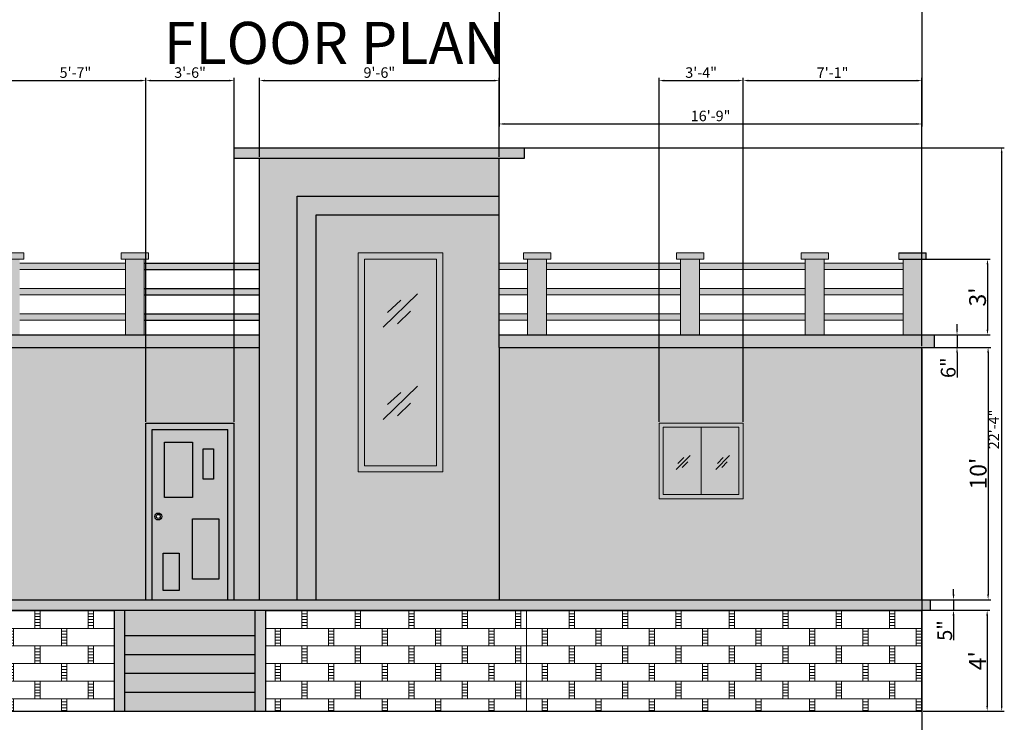
# Model space of a CAD drawing. Units: inches. Extents: x 1662 to 23131, y 1265 to 19127.
# Tile 23 of 26: x 22111 to 22579, y 18027 to 18361. Entities that reach past the tile are written whole.
import ezdxf

# ---------------------------------------------------------------- set-up
doc = ezdxf.new("R2010")
doc.units = ezdxf.units.IN
for name, color, linetype, lineweight in [('A-ANNO-DIMS', 4, 'Continuous', 18), ('A-ANNO-TITL', 7, 'Continuous', 35), ('A-ELEV', 7, 'Continuous', 25), ('A-ELEV-GLAZ', 4, 'Continuous', 18), ('A-ELEV-PATT', 8, 'Continuous', 13), ('A-ELEV-RAIL', 7, 'Continuous', 18), ('A-ELEV-SURF-PATT', 252, 'Continuous', 13)]:
    doc.layers.add(name, color=color, linetype=linetype, lineweight=lineweight)
doc.styles.get("Standard").update_dxf_attribs({"font": 'arial.ttf'})
doc.dimstyles.new('ISO-25', dxfattribs={"dimtxt": 5, "dimasz": 2.5, "dimexe": 1.25, "dimexo": 0.625, "dimtad": 1, "dimlunit": 3, "dimtxsty": 'Standard', "dimcen": 2.5, "dimadec": 0, "dimazin": 0, "dimtfac": 1, "dimtmove": 0, "dimatfit": 3, "dimfxl": 1, "dimarcsym": 0})

# ---------------------------------------------------------------- blocks, each defined once
blk = doc.blocks.new('*D137')
at = {"layer": 'A-ANNO-DIMS', "color": 0, "lineweight": -2, "transparency": 16777216}
for p, q in [((22540.77, 18080.22), (22572.4, 18080.22)), ((22571.15, 18077.72), (22571.15, 18034.72)), ((22540.77, 18032.22), (22572.4, 18032.22))]:
    blk.add_line(p, q, dxfattribs=at)
at = {"layer": 'A-ANNO-DIMS', "color": 0, "transparency": 16777216}
for points in [[(22570.74, 18077.72), (22571.57, 18077.72), (22571.15, 18080.22)], [(22570.74, 18034.72), (22571.57, 18034.72), (22571.15, 18032.22)]]:
    blk.add_solid(points, dxfattribs=at)
at = {"layer": 'Defpoints', "color": 0, "transparency": 16777216}
for p in [(22540.15, 18080.22), (22540.15, 18032.22), (22571.15, 18032.22)]:
    blk.add_point(p, dxfattribs=at)
at = {"layer": 'A-ANNO-DIMS', "color": 0, "transparency": 16777216, "insert": (22566.53, 18056.22), "char_height": 5, "attachment_point": 5, "rotation": 90}
blk.add_mtext("{\\H1.6x;4'}", dxfattribs=at)
blk = doc.blocks.new('*D138')
at = {"layer": 'A-ANNO-DIMS', "color": 0, "lineweight": -2, "transparency": 16777216}
for p, q in [((22555.15, 18087.72), (22555.15, 18090.22)), ((22544.77, 18085.22), (22556.4, 18085.22)), ((22555.15, 18085.22), (22555.15, 18080.22)), ((22544.77, 18080.22), (22556.4, 18080.22)), ((22555.15, 18077.72), (22555.15, 18065.93))]:
    blk.add_line(p, q, dxfattribs=at)
at = {"layer": 'A-ANNO-DIMS', "color": 0, "transparency": 16777216}
for points in [[(22554.73, 18087.72), (22555.57, 18087.72), (22555.15, 18085.22)], [(22554.73, 18077.72), (22555.57, 18077.72), (22555.15, 18080.22)]]:
    blk.add_solid(points, dxfattribs=at)
at = {"layer": 'Defpoints', "color": 0, "transparency": 16777216}
for p in [(22544.15, 18085.22), (22544.15, 18080.22), (22555.15, 18080.22)]:
    blk.add_point(p, dxfattribs=at)
at = {"layer": 'A-ANNO-DIMS', "color": 0, "transparency": 16777216, "insert": (22550.97, 18070.57), "char_height": 5, "attachment_point": 5, "rotation": 90}
blk.add_mtext('{\\H1.4x;5"}', dxfattribs=at)
blk = doc.blocks.new('*D139')
at = {"layer": 'A-ANNO-DIMS', "color": 0, "lineweight": -2, "transparency": 16777216}
for p, q in [((22540.77, 18205.22), (22572.85, 18205.22)), ((22571.6, 18202.72), (22571.6, 18087.72)), ((22540.77, 18085.22), (22572.85, 18085.22))]:
    blk.add_line(p, q, dxfattribs=at)
at = {"layer": 'A-ANNO-DIMS', "color": 0, "transparency": 16777216}
for points in [[(22571.18, 18202.72), (22572.02, 18202.72), (22571.6, 18205.22)], [(22571.18, 18087.72), (22572.02, 18087.72), (22571.6, 18085.22)]]:
    blk.add_solid(points, dxfattribs=at)
at = {"layer": 'Defpoints', "color": 0, "transparency": 16777216}
for p in [(22540.15, 18205.22), (22540.15, 18085.22), (22571.6, 18085.22)]:
    blk.add_point(p, dxfattribs=at)
at = {"layer": 'A-ANNO-DIMS', "color": 0, "transparency": 16777216, "insert": (22566.89, 18145.22), "char_height": 5, "attachment_point": 5, "rotation": 90}
blk.add_mtext("{\\H1.6x;10'}", dxfattribs=at)
blk = doc.blocks.new('*D140')
at = {"layer": 'A-ANNO-DIMS', "color": 0, "lineweight": -2, "transparency": 16777216}
for p, q in [((22556.81, 18213.72), (22556.81, 18216.22)), ((22546.77, 18211.22), (22558.06, 18211.22)), ((22556.81, 18211.22), (22556.81, 18205.22)), ((22546.77, 18205.22), (22558.06, 18205.22)), ((22556.81, 18202.72), (22556.81, 18190.89))]:
    blk.add_line(p, q, dxfattribs=at)
at = {"layer": 'A-ANNO-DIMS', "color": 0, "transparency": 16777216}
for points in [[(22556.4, 18213.72), (22557.23, 18213.72), (22556.81, 18211.22)], [(22556.4, 18202.72), (22557.23, 18202.72), (22556.81, 18205.22)]]:
    blk.add_solid(points, dxfattribs=at)
at = {"layer": 'Defpoints', "color": 0, "transparency": 16777216}
for p in [(22546.15, 18211.22), (22546.15, 18205.22), (22556.81, 18205.22)]:
    blk.add_point(p, dxfattribs=at)
at = {"layer": 'A-ANNO-DIMS', "color": 0, "transparency": 16777216, "insert": (22552.61, 18195.56), "char_height": 5, "attachment_point": 5, "rotation": 90}
blk.add_mtext('{\\H1.4x;6"}', dxfattribs=at)
blk = doc.blocks.new('*D141')
at = {"layer": 'A-ANNO-DIMS', "color": 0, "lineweight": -2, "transparency": 16777216}
for p, q in [((22540.77, 18247.22), (22572.55, 18247.22)), ((22571.3, 18244.72), (22571.3, 18213.72)), ((22540.77, 18211.22), (22572.55, 18211.22))]:
    blk.add_line(p, q, dxfattribs=at)
at = {"layer": 'A-ANNO-DIMS', "color": 0, "transparency": 16777216}
for points in [[(22570.88, 18244.72), (22571.71, 18244.72), (22571.3, 18247.22)], [(22570.88, 18213.72), (22571.71, 18213.72), (22571.3, 18211.22)]]:
    blk.add_solid(points, dxfattribs=at)
at = {"layer": 'Defpoints', "color": 0, "transparency": 16777216}
for p in [(22540.15, 18247.22), (22540.15, 18211.22), (22571.3, 18211.22)]:
    blk.add_point(p, dxfattribs=at)
at = {"layer": 'A-ANNO-DIMS', "color": 0, "transparency": 16777216, "insert": (22566.58, 18229.22), "char_height": 5, "attachment_point": 5, "rotation": 90}
blk.add_mtext("{\\H1.6x;3'}", dxfattribs=at)
blk = doc.blocks.new('GLAZ-REFLECTION')
for p, q in [((0, 0), (6.63, 6.69)), ((0.83, 2.91), (3.6, 5.77)), ((2.93, 0.98), (5.5, 3.58))]:
    blk.add_line(p, q)
blk = doc.blocks.new('*D255')
at = {"layer": 'A-ANNO-DIMS', "color": 0, "lineweight": -2, "transparency": 16777216}
for p, q in [((22339.15, 18570.08), (22339.15, 18310.24)), ((22540.15, 18570.08), (22540.15, 18310.24)), ((22341.65, 18311.49), (22537.65, 18311.49))]:
    blk.add_line(p, q, dxfattribs=at)
at = {"layer": 'A-ANNO-DIMS', "color": 0, "transparency": 16777216}
for points in [[(22341.65, 18311.91), (22341.65, 18311.08), (22339.15, 18311.49)], [(22537.65, 18311.91), (22537.65, 18311.08), (22540.15, 18311.49)]]:
    blk.add_solid(points, dxfattribs=at)
at = {"layer": 'Defpoints', "color": 0, "transparency": 16777216}
for p in [(22339.15, 18570.71), (22540.15, 18570.71), (22540.15, 18311.49)]:
    blk.add_point(p, dxfattribs=at)
at = {"layer": 'A-ANNO-DIMS', "color": 0, "transparency": 16777216, "insert": (22439.65, 18314.67), "char_height": 5, "attachment_point": 5}
blk.add_mtext('16\'-9"', dxfattribs=at)
blk = doc.blocks.new('*D257')
at = {"layer": 'A-ANNO-DIMS', "color": 0, "lineweight": -2, "transparency": 16777216}
for p, q in [((21988.15, 18204.6), (21988.15, 17831.29)), ((22540.15, 18204.6), (22540.15, 17831.29)), ((21990.65, 17832.54), (22537.65, 17832.54))]:
    blk.add_line(p, q, dxfattribs=at)
at = {"layer": 'A-ANNO-DIMS', "color": 0, "transparency": 16777216}
for points in [[(21990.65, 17832.96), (21990.65, 17832.12), (21988.15, 17832.54)], [(22537.65, 17832.96), (22537.65, 17832.12), (22540.15, 17832.54)]]:
    blk.add_solid(points, dxfattribs=at)
at = {"layer": 'Defpoints', "color": 0, "transparency": 16777216}
for p in [(21988.15, 18205.22), (22540.15, 18205.22), (22540.15, 17832.54)]:
    blk.add_point(p, dxfattribs=at)
at = {"layer": 'A-ANNO-DIMS', "color": 0, "transparency": 16777216, "insert": (22264.15, 17835.72), "char_height": 5, "attachment_point": 5}
blk.add_mtext('46\'-0"', dxfattribs=at)
blk = doc.blocks.new('*D258')
at = {"layer": 'A-ANNO-DIMS', "color": 0, "lineweight": -2, "transparency": 16777216}
for p, q in [((22213.77, 18300.22), (22579.3, 18300.22)), ((22578.05, 18034.72), (22578.05, 18297.72)), ((22540.77, 18032.22), (22579.3, 18032.22))]:
    blk.add_line(p, q, dxfattribs=at)
at = {"layer": 'A-ANNO-DIMS', "color": 0, "transparency": 16777216}
for points in [[(22577.63, 18297.72), (22578.47, 18297.72), (22578.05, 18300.22)], [(22577.63, 18034.72), (22578.47, 18034.72), (22578.05, 18032.22)]]:
    blk.add_solid(points, dxfattribs=at)
at = {"layer": 'Defpoints', "color": 0, "transparency": 16777216}
for p in [(22213.15, 18300.22), (22578.05, 18300.22), (22540.15, 18032.22)]:
    blk.add_point(p, dxfattribs=at)
at = {"layer": 'A-ANNO-DIMS', "color": 0, "transparency": 16777216, "insert": (22574.91, 18166.22), "char_height": 5, "attachment_point": 5, "rotation": 90}
blk.add_mtext('22\'-4"', dxfattribs=at)
blk = doc.blocks.new('*D261')
at = {"layer": 'A-ANNO-DIMS', "color": 0, "lineweight": -2, "transparency": 16777216}
for p, q in [((22104.15, 18169.85), (22104.15, 18333.37)), ((22171.15, 18169.85), (22171.15, 18333.37)), ((22106.65, 18332.12), (22168.65, 18332.12))]:
    blk.add_line(p, q, dxfattribs=at)
at = {"layer": 'A-ANNO-DIMS', "color": 0, "transparency": 16777216}
for points in [[(22106.65, 18332.54), (22106.65, 18331.71), (22104.15, 18332.12)], [(22168.65, 18332.54), (22168.65, 18331.71), (22171.15, 18332.12)]]:
    blk.add_solid(points, dxfattribs=at)
at = {"layer": 'Defpoints', "color": 0, "transparency": 16777216}
for p in [(22171.15, 18332.12), (22104.15, 18169.22), (22171.15, 18169.22)]:
    blk.add_point(p, dxfattribs=at)
at = {"layer": 'A-ANNO-DIMS', "color": 0, "transparency": 16777216, "insert": (22137.65, 18335.29), "char_height": 5, "attachment_point": 5}
blk.add_mtext('5\'-7"', dxfattribs=at)
blk = doc.blocks.new('*D262')
at = {"layer": 'A-ANNO-DIMS', "color": 0, "lineweight": -2, "transparency": 16777216}
for p, q in [((22171.15, 18169.85), (22171.15, 18333.37)), ((22213.15, 18169.85), (22213.15, 18333.37)), ((22173.65, 18332.12), (22210.65, 18332.12))]:
    blk.add_line(p, q, dxfattribs=at)
at = {"layer": 'A-ANNO-DIMS', "color": 0, "transparency": 16777216}
for points in [[(22173.65, 18332.54), (22173.65, 18331.71), (22171.15, 18332.12)], [(22210.65, 18332.54), (22210.65, 18331.71), (22213.15, 18332.12)]]:
    blk.add_solid(points, dxfattribs=at)
at = {"layer": 'Defpoints', "color": 0, "transparency": 16777216}
for p in [(22213.15, 18332.12), (22171.15, 18169.22), (22213.15, 18169.22)]:
    blk.add_point(p, dxfattribs=at)
at = {"layer": 'A-ANNO-DIMS', "color": 0, "transparency": 16777216, "insert": (22192.15, 18335.3), "char_height": 5, "attachment_point": 5}
blk.add_mtext('3\'-6"', dxfattribs=at)
blk = doc.blocks.new('*D263')
at = {"layer": 'A-ANNO-DIMS', "color": 0, "lineweight": -2, "transparency": 16777216}
for p, q in [((22225.15, 18295.85), (22225.15, 18333.37)), ((22339.15, 18295.85), (22339.15, 18333.37)), ((22227.65, 18332.12), (22336.65, 18332.12))]:
    blk.add_line(p, q, dxfattribs=at)
at = {"layer": 'A-ANNO-DIMS', "color": 0, "transparency": 16777216}
for points in [[(22227.65, 18332.54), (22227.65, 18331.71), (22225.15, 18332.12)], [(22336.65, 18332.54), (22336.65, 18331.71), (22339.15, 18332.12)]]:
    blk.add_solid(points, dxfattribs=at)
at = {"layer": 'Defpoints', "color": 0, "transparency": 16777216}
for p in [(22339.15, 18332.12), (22225.15, 18295.22), (22339.15, 18295.22)]:
    blk.add_point(p, dxfattribs=at)
at = {"layer": 'A-ANNO-DIMS', "color": 0, "transparency": 16777216, "insert": (22282.15, 18335.3), "char_height": 5, "attachment_point": 5}
blk.add_mtext('9\'-6"', dxfattribs=at)
blk = doc.blocks.new('*D264')
at = {"layer": 'A-ANNO-DIMS', "color": 0, "lineweight": -2, "transparency": 16777216}
for p, q in [((22415.15, 18169.85), (22415.15, 18333.37)), ((22455.15, 18169.85), (22455.15, 18333.37)), ((22417.65, 18332.12), (22452.65, 18332.12))]:
    blk.add_line(p, q, dxfattribs=at)
at = {"layer": 'A-ANNO-DIMS', "color": 0, "transparency": 16777216}
for points in [[(22417.65, 18332.54), (22417.65, 18331.71), (22415.15, 18332.12)], [(22452.65, 18332.54), (22452.65, 18331.71), (22455.15, 18332.12)]]:
    blk.add_solid(points, dxfattribs=at)
at = {"layer": 'Defpoints', "color": 0, "transparency": 16777216}
for p in [(22455.15, 18332.12), (22415.15, 18169.22), (22455.15, 18169.22)]:
    blk.add_point(p, dxfattribs=at)
at = {"layer": 'A-ANNO-DIMS', "color": 0, "transparency": 16777216, "insert": (22435.15, 18335.3), "char_height": 5, "attachment_point": 5}
blk.add_mtext('3\'-4"', dxfattribs=at)
blk = doc.blocks.new('*D265')
at = {"layer": 'A-ANNO-DIMS', "color": 0, "lineweight": -2, "transparency": 16777216}
for p, q in [((22455.15, 18169.85), (22455.15, 18333.37)), ((22540.15, 18205.85), (22540.15, 18333.37)), ((22457.65, 18332.12), (22537.65, 18332.12))]:
    blk.add_line(p, q, dxfattribs=at)
at = {"layer": 'A-ANNO-DIMS', "color": 0, "transparency": 16777216}
for points in [[(22457.65, 18332.54), (22457.65, 18331.71), (22455.15, 18332.12)], [(22537.65, 18332.54), (22537.65, 18331.71), (22540.15, 18332.12)]]:
    blk.add_solid(points, dxfattribs=at)
at = {"layer": 'Defpoints', "color": 0, "transparency": 16777216}
for p in [(22540.15, 18332.12), (22540.15, 18205.22), (22455.15, 18169.22)]:
    blk.add_point(p, dxfattribs=at)
at = {"layer": 'A-ANNO-DIMS', "color": 0, "transparency": 16777216, "insert": (22497.65, 18335.26), "char_height": 5, "attachment_point": 5}
blk.add_mtext('7\'-1"', dxfattribs=at)

msp = doc.modelspace()

# ---------------------------------------------------------------- hatches: boundary and pattern name
at = {"layer": 'A-ELEV-PATT'}
h = msp.add_hatch(dxfattribs=at)
h.set_pattern_fill('BRSTONE', color=256)
h.paths.add_polyline_path([(22156.149, 18080.223), (22079.649, 18080.223), (22079.649, 18032.223), (22156.149, 18032.223)])
h.paths.add_polyline_path([(22079.649, 18080.223), (22048.849, 18080.223), (22049.648, 18077.151), (22046.197, 18075.676), (22049.648, 18074.202), (22051.373, 18060.93), (22047.922, 18055.032), (22052.523, 18054.294), (22053.673, 18052.082), (22050.798, 18046.921), (22055.399, 18043.972), (22050.798, 18039.548), (22053.673, 18039.548), (22058.118, 18032.223), (22079.649, 18032.223)])
h.paths.add_polyline_path([(21997.887, 18071.252), (22000.763, 18076.413), (22004.213, 18077.151), (22004.746, 18080.223), (21988.149, 18080.223), (21988.149, 18042.556), (21991.561, 18047.659), (21992.711, 18055.032), (21990.986, 18056.506), (21994.436, 18064.617), (21998.462, 18065.354)])
h = msp.add_hatch(dxfattribs=at)
h.set_pattern_fill('AR-BRSTD', color=256)
h.paths.add_polyline_path([(22339.149, 18080.223), (22228.149, 18080.223), (22228.149, 18032.223), (22339.149, 18032.223)])
h.paths.add_polyline_path([(22540.149, 18080.223), (22339.149, 18080.223), (22339.149, 18032.223), (22540.149, 18032.223)])
h = msp.add_hatch(dxfattribs=at)
h.set_pattern_fill('AR-BRSTD', color=256)
h.paths.add_polyline_path([(22540.149, 18080.223), (22228.149, 18080.223), (22228.149, 18032.223), (22540.149, 18032.223)])
h = msp.add_hatch(dxfattribs=at)
h.set_pattern_fill('BRSTONE', color=256)
h.paths.add_polyline_path([(22540.149, 18080.223), (22228.149, 18080.223), (22228.149, 18032.223), (22540.149, 18032.223)])
at = {"layer": 'A-ELEV-SURF-PATT'}
h = msp.add_hatch(color=256, dxfattribs=at)
h.dxf.hatch_style = 1
h.paths.add_polyline_path([(22225.149, 18211.223), (21982.149, 18211.223), (21982.149, 18205.223), (22225.149, 18205.223)])
h.paths.add_polyline_path([(22546.149, 18211.223), (22339.149, 18211.223), (22339.149, 18205.223), (22546.149, 18205.223)])
h.paths.add_polyline_path([(22351.149, 18300.223), (22213.149, 18300.223), (22213.149, 18295.223), (22351.149, 18295.223)])
h = msp.add_hatch(color=256, dxfattribs=at)
h.dxf.hatch_style = 1
h.paths.add_polyline_path([(22225.149, 18205.223), (21988.149, 18205.223), (21988.149, 18085.223), (22005.644, 18085.223), (22005.939, 18086.736), (22001.913, 18091.16), (22005.364, 18094.109), (22013.415, 18103.694), (22012.84, 18106.643), (22017.441, 18108.855), (22015.141, 18109.592), (22013.415, 18113.279), (22020.317, 18119.177), (22024.343, 18128.025), (22026.643, 18122.126), (22027.793, 18123.601), (22031.244, 18114.016), (22032.969, 18115.491), (22037.57, 18103.694), (22039.296, 18106.643), (22043.321, 18098.533), (22041.596, 18089.685), (22046.772, 18088.21), (22047.549, 18085.223), (22171.149, 18085.223), (22171.149, 18169.223), (22213.149, 18169.223), (22213.149, 18085.223), (22225.149, 18085.223)])
h.paths.add_polyline_path([(22064.149, 18169.223), (22104.149, 18169.223), (22104.149, 18133.223), (22064.149, 18133.223)], flags=16)
h.paths.add_polyline_path([(22066.149, 18167.223), (22102.149, 18167.223), (22102.149, 18135.223), (22066.149, 18135.223)], flags=0)
h.paths.add_polyline_path([(22540.149, 18205.223), (22339.149, 18205.223), (22339.149, 18085.223), (22540.149, 18085.223)])
h.paths.add_polyline_path([(22415.149, 18169.223), (22455.149, 18169.223), (22455.149, 18133.223), (22415.149, 18133.223)], flags=16)
h.paths.add_polyline_path([(22417.149, 18167.223), (22453.149, 18167.223), (22453.149, 18135.223), (22417.149, 18135.223)], flags=0)
h.paths.add_polyline_path([(22339.149, 18205.223), (22339.149, 18268.223), (22252.149, 18268.223), (22252.149, 18211.223), (22252.149, 18085.223), (22339.149, 18085.223)], flags=17)
h.paths.add_polyline_path([(22272.061, 18145.984), (22272.061, 18250.207), (22312.36, 18250.207), (22312.36, 18145.984)], flags=16)
h.paths.add_polyline_path([(22275.061, 18148.984), (22275.061, 18247.207), (22309.36, 18247.207), (22309.36, 18148.984)], flags=0)
h.paths.add_polyline_path([(22243.149, 18211.223), (22243.149, 18277.223), (22339.149, 18277.223), (22339.149, 18295.223), (22225.149, 18295.223), (22225.149, 18211.223), (22225.149, 18085.223), (22243.149, 18085.223)])
h = msp.add_hatch(color=256, dxfattribs=at)
h.dxf.hatch_style = 1
h.paths.add_polyline_path([(22252.149, 18211.223), (22252.149, 18268.223), (22339.149, 18268.223), (22339.149, 18277.223), (22243.149, 18277.223), (22243.149, 18211.223), (22243.149, 18085.223), (22252.149, 18085.223)])
h = msp.add_hatch(color=256, dxfattribs=at)
h.dxf.hatch_style = 1
h.paths.add_polyline_path([(21999.149, 18250.223), (21986.149, 18250.223), (21986.149, 18247.223), (21999.149, 18247.223)])
h.paths.add_polyline_path([(22053.899, 18250.223), (22040.899, 18250.223), (22040.899, 18247.223), (22053.899, 18247.223)])
h.paths.add_polyline_path([(22113.149, 18250.223), (22100.149, 18250.223), (22100.149, 18247.223), (22113.149, 18247.223)])
h.paths.add_polyline_path([(22172.399, 18250.223), (22159.399, 18250.223), (22159.399, 18247.223), (22172.399, 18247.223)])
h.paths.add_polyline_path([(22363.649, 18250.223), (22350.649, 18250.223), (22350.649, 18247.223), (22363.649, 18247.223)])
h.paths.add_polyline_path([(22436.399, 18250.223), (22423.399, 18250.223), (22423.399, 18247.223), (22436.399, 18247.223)])
h.paths.add_polyline_path([(22495.649, 18250.223), (22482.649, 18250.223), (22482.649, 18247.223), (22495.649, 18247.223)])
h.paths.add_polyline_path([(22542.149, 18250.223), (22529.149, 18250.223), (22529.149, 18247.223), (22542.149, 18247.223)])
h = msp.add_hatch(color=256, dxfattribs=at)
h.dxf.hatch_style = 1
h.paths.add_polyline_path([(22104.149, 18169.223), (22064.149, 18169.223), (22064.149, 18133.223), (22104.149, 18133.223)])
h.paths.add_polyline_path([(22102.149, 18167.223), (22102.149, 18135.223), (22066.149, 18135.223), (22066.149, 18167.223)], flags=16)
h.paths.add_polyline_path([(22455.149, 18169.223), (22415.149, 18169.223), (22415.149, 18133.223), (22455.149, 18133.223)])
h.paths.add_polyline_path([(22453.149, 18167.223), (22453.149, 18135.223), (22417.149, 18135.223), (22417.149, 18167.223)], flags=16)
h.paths.add_polyline_path([(22312.36, 18250.207), (22272.061, 18250.207), (22272.061, 18145.984), (22312.36, 18145.984)])
h.paths.add_polyline_path([(22309.36, 18148.984), (22275.061, 18148.984), (22275.061, 18247.207), (22309.36, 18247.207)], flags=16)
h.paths.add_polyline_path([(22042.899, 18245.223), (21997.149, 18245.223), (21997.149, 18242.223), (22042.899, 18242.223)])
h.paths.add_polyline_path([(22042.899, 18233.223), (21997.149, 18233.223), (21997.149, 18230.223), (22042.899, 18230.223)])
h.paths.add_polyline_path([(22042.899, 18221.223), (21997.149, 18221.223), (21997.149, 18218.223), (22042.899, 18218.223)])
h.paths.add_polyline_path([(22102.149, 18221.223), (22051.899, 18221.223), (22051.899, 18218.223), (22102.149, 18218.223)])
h.paths.add_polyline_path([(22102.149, 18233.223), (22051.899, 18233.223), (22051.899, 18230.223), (22102.149, 18230.223)])
h.paths.add_polyline_path([(22102.149, 18245.223), (22051.899, 18245.223), (22051.899, 18242.223), (22102.149, 18242.223)])
h.paths.add_polyline_path([(22161.399, 18245.223), (22111.149, 18245.223), (22111.149, 18242.223), (22161.399, 18242.223)])
h.paths.add_polyline_path([(22161.399, 18233.223), (22111.149, 18233.223), (22111.149, 18230.223), (22161.399, 18230.223)])
h.paths.add_polyline_path([(22161.399, 18221.223), (22111.149, 18221.223), (22111.149, 18218.223), (22161.399, 18218.223)])
h.paths.add_polyline_path([(22225.149, 18221.223), (22170.399, 18221.223), (22170.399, 18218.223), (22225.149, 18218.223)])
h.paths.add_polyline_path([(22225.149, 18233.223), (22170.399, 18233.223), (22170.399, 18230.223), (22225.149, 18230.223)])
h.paths.add_polyline_path([(22225.149, 18245.223), (22170.399, 18245.223), (22170.399, 18242.223), (22225.149, 18242.223)])
h.paths.add_polyline_path([(22352.649, 18233.223), (22339.149, 18233.223), (22339.149, 18230.223), (22352.649, 18230.223)])
h.paths.add_polyline_path([(22352.649, 18221.223), (22339.149, 18221.223), (22339.149, 18218.223), (22352.649, 18218.223)])
h.paths.add_polyline_path([(22352.649, 18245.223), (22339.149, 18245.223), (22339.149, 18242.223), (22352.649, 18242.223)])
h.paths.add_polyline_path([(22425.399, 18245.223), (22361.649, 18245.223), (22361.649, 18242.223), (22425.399, 18242.223)])
h.paths.add_polyline_path([(22425.399, 18233.223), (22361.649, 18233.223), (22361.649, 18230.223), (22425.399, 18230.223)])
h.paths.add_polyline_path([(22425.399, 18221.223), (22361.649, 18221.223), (22361.649, 18218.223), (22425.399, 18218.223)])
h.paths.add_polyline_path([(22484.649, 18245.223), (22434.399, 18245.223), (22434.399, 18242.223), (22484.649, 18242.223)])
h.paths.add_polyline_path([(22484.649, 18233.223), (22434.399, 18233.223), (22434.399, 18230.223), (22484.649, 18230.223)])
h.paths.add_polyline_path([(22484.649, 18221.223), (22434.399, 18221.223), (22434.399, 18218.223), (22484.649, 18218.223)])
h.paths.add_polyline_path([(22531.149, 18221.223), (22493.649, 18221.223), (22493.649, 18218.223), (22531.149, 18218.223)])
h.paths.add_polyline_path([(22531.149, 18233.223), (22493.649, 18233.223), (22493.649, 18230.223), (22531.149, 18230.223)])
h.paths.add_polyline_path([(22531.149, 18245.223), (22493.649, 18245.223), (22493.649, 18242.223), (22531.149, 18242.223)])
h = msp.add_hatch(color=256, dxfattribs=at)
h.dxf.hatch_style = 1
h.paths.add_polyline_path([(22493.649, 18247.223), (22484.649, 18247.223), (22484.649, 18211.223), (22493.649, 18211.223)])
h.paths.add_polyline_path([(22434.399, 18247.223), (22425.399, 18247.223), (22425.399, 18211.223), (22434.399, 18211.223)])
h.paths.add_polyline_path([(22361.649, 18247.223), (22352.649, 18247.223), (22352.649, 18211.223), (22361.649, 18211.223)])
h.paths.add_polyline_path([(22170.399, 18247.223), (22161.399, 18247.223), (22161.399, 18211.223), (22170.399, 18211.223)])
h.paths.add_polyline_path([(22111.149, 18247.223), (22102.149, 18247.223), (22102.149, 18211.223), (22111.149, 18211.223)])
h.paths.add_polyline_path([(22051.899, 18247.223), (22042.899, 18247.223), (22042.899, 18211.223), (22051.899, 18211.223)])
h.paths.add_polyline_path([(21997.149, 18247.223), (21988.149, 18247.223), (21988.149, 18211.223), (21997.149, 18211.223)])
h = msp.add_hatch(color=256, dxfattribs=at)
h.dxf.hatch_style = 1
h.paths.add_polyline_path([(22309.36, 18247.207), (22275.061, 18247.207), (22275.061, 18148.984), (22309.36, 18148.984)])
h = msp.add_hatch(color=256, dxfattribs=at)
h.dxf.hatch_style = 1
h.paths.add_polyline_path([(22540.149, 18247.223), (22531.149, 18247.223), (22531.149, 18211.223), (22540.149, 18211.223)])
h = msp.add_hatch(color=256, dxfattribs=at)
h.dxf.hatch_style = 1
h.paths.add_polyline_path([(22161.149, 18080.223), (22156.149, 18080.223), (22156.149, 18032.223), (22161.149, 18032.223)])
h.paths.add_polyline_path([(22228.149, 18080.223), (22223.149, 18080.223), (22223.149, 18032.223), (22228.149, 18032.223)])
h.paths.add_polyline_path([(22213.149, 18169.223), (22171.149, 18169.223), (22171.149, 18085.223), (22174.149, 18085.223), (22174.149, 18166.223), (22210.149, 18166.223), (22210.149, 18085.223), (22213.149, 18085.223)])
h = msp.add_hatch(color=256, dxfattribs=at)
h.dxf.hatch_style = 1
h.paths.add_polyline_path([(22084.149, 18167.223), (22066.149, 18167.223), (22066.149, 18135.223), (22084.149, 18135.223)])
h.paths.add_polyline_path([(22102.149, 18167.223), (22084.149, 18167.223), (22084.149, 18135.223), (22102.149, 18135.223)])
h.paths.add_polyline_path([(22435.149, 18167.223), (22417.149, 18167.223), (22417.149, 18135.223), (22435.149, 18135.223)])
h.paths.add_polyline_path([(22453.149, 18167.223), (22435.149, 18167.223), (22435.149, 18135.223), (22453.149, 18135.223)])
h = msp.add_hatch(color=256, dxfattribs=at)
h.dxf.hatch_style = 1
h.paths.add_polyline_path([(22210.149, 18166.223), (22174.149, 18166.223), (22174.149, 18085.223), (22210.149, 18085.223)])
h.paths.add_polyline_path([(22175.383, 18124.82, -1), (22178.687, 18124.82, -1)], flags=16)
h.paths.add_polyline_path([(22176.08, 18124.82, -1), (22177.99, 18124.82, -1)], flags=0)
h.paths.add_polyline_path([(22193.376, 18123.759), (22205.819, 18123.759), (22205.819, 18094.971), (22193.376, 18094.971)], flags=16)
h.paths.add_polyline_path([(22180.056, 18133.813), (22180.056, 18160.203), (22193.373, 18160.203), (22193.373, 18133.813)], flags=16)
h.paths.add_polyline_path([(22186.961, 18107.343), (22186.961, 18089.624), (22179.399, 18089.624), (22179.399, 18107.343)], flags=16)
h.paths.add_polyline_path([(22198.399, 18142.531), (22198.399, 18157.022), (22203.234, 18157.022), (22203.234, 18142.531)], flags=16)
h = msp.add_hatch(color=256, dxfattribs=at)
h.dxf.hatch_style = 1
h.paths.add_polyline_path([(22193.373, 18160.203), (22180.056, 18160.203), (22180.056, 18133.813), (22193.373, 18133.813)])
h.paths.add_polyline_path([(22203.234, 18157.022), (22198.399, 18157.022), (22198.399, 18142.531), (22203.234, 18142.531)])
h.paths.add_polyline_path([(22205.819, 18123.759), (22193.376, 18123.759), (22193.376, 18094.971), (22205.819, 18094.971)])
h.paths.add_polyline_path([(22186.961, 18107.343), (22179.399, 18107.343), (22179.399, 18089.624), (22186.961, 18089.624)])
h = msp.add_hatch(color=256, dxfattribs=at)
h.dxf.hatch_style = 1
h.paths.add_polyline_path([(22544.149, 18085.223), (22047.549, 18085.223), (22048.849, 18080.223), (22544.149, 18080.223)])
h.paths.add_polyline_path([(22005.364, 18083.787), (22005.644, 18085.223), (21984.149, 18085.223), (21984.149, 18080.223), (22004.746, 18080.223)])
h = msp.add_hatch(color=256, dxfattribs=at)
h.dxf.hatch_style = 1
h.paths.add_polyline_path([(22223.149, 18041.223), (22161.149, 18041.223), (22161.149, 18032.223), (22223.149, 18032.223)])
h.paths.add_polyline_path([(22223.149, 18050.223), (22161.149, 18050.223), (22161.149, 18041.223), (22223.149, 18041.223)])
h.paths.add_polyline_path([(22223.149, 18059.223), (22161.149, 18059.223), (22161.149, 18050.223), (22223.149, 18050.223)])
h.paths.add_polyline_path([(22223.149, 18068.223), (22161.149, 18068.223), (22161.149, 18059.223), (22223.149, 18059.223)])
h.paths.add_polyline_path([(22223.149, 18080.223), (22161.149, 18080.223), (22161.149, 18068.223), (22223.149, 18068.223)])

# ---------------------------------------------------------------- linework, layer by layer
at = {"layer": 'A-ELEV'}
for p, q in [((22213.149, 18300.223), (22351.149, 18300.223)), ((22213.149, 18295.223), (22213.149, 18300.223)), ((22351.149, 18295.223), (22351.149, 18300.223)), ((22213.149, 18295.223), (22351.149, 18295.223)), ((22225.149, 18211.223), (22225.149, 18295.223)), ((22339.149, 18205.223), (22339.149, 18295.223)), ((22243.149, 18211.223), (22243.149, 18277.223)), ((22243.149, 18277.223), (22339.149, 18277.223)), ((22252.149, 18268.223), (22339.149, 18268.223)), ((22252.149, 18211.223), (22252.149, 18268.223)), ((22529.149, 18250.223), (22542.149, 18250.223)), ((22542.149, 18247.223), (22542.149, 18250.223)), ((22542.149, 18247.223), (22542.149, 18250.223)), ((22170.399, 18245.223), (22225.149, 18245.223)), ((22529.149, 18247.223), (22542.149, 18247.223)), ((22170.399, 18242.223), (22225.149, 18242.223)), ((22170.399, 18233.223), (22225.149, 18233.223)), ((22170.399, 18230.223), (22225.149, 18230.223)), ((22284.024, 18214.824), (22300.327, 18230.638)), ((22286.033, 18221.905), (22292.412, 18227.687)), ((22170.399, 18221.223), (22225.149, 18221.223)), ((22290.758, 18216.476), (22296.901, 18222.495)), ((22170.399, 18218.223), (22225.149, 18218.223)), ((21982.149, 18211.223), (22225.149, 18211.223)), ((22225.149, 18085.223), (22225.149, 18211.223)), ((22243.149, 18085.223), (22243.149, 18211.223)), ((22252.149, 18085.223), (22252.149, 18211.223)), ((22339.149, 18205.223), (22339.149, 18211.223)), ((22339.149, 18211.223), (22546.149, 18211.223)), ((22546.149, 18205.223), (22546.149, 18211.223)), ((21982.149, 18205.223), (22225.149, 18205.223)), ((22339.149, 18205.223), (22339.149, 18085.223)), ((22339.149, 18205.223), (22546.149, 18205.223)), ((22540.149, 18085.223), (22540.149, 18205.223)), ((22284.024, 18170.972), (22300.327, 18186.787)), ((22286.033, 18178.053), (22292.412, 18183.836)), ((22290.758, 18172.625), (22296.901, 18178.643)), ((22171.149, 18085.223), (22171.149, 18169.223)), ((22171.149, 18169.223), (22213.149, 18169.223)), ((22213.149, 18085.223), (22213.149, 18169.223)), ((22174.149, 18085.223), (22174.149, 18166.223)), ((22174.149, 18166.223), (22210.149, 18166.223)), ((22210.149, 18085.223), (22210.149, 18166.223)), ((22047.549, 18085.223), (22544.149, 18085.223)), ((22544.149, 18080.223), (22544.149, 18085.223)), ((22048.849, 18080.223), (22544.149, 18080.223)), ((22156.149, 18032.223), (22156.149, 18080.223)), ((22161.149, 18032.223), (22161.149, 18080.223)), ((22223.149, 18032.223), (22223.149, 18080.223)), ((22228.149, 18032.223), (22228.149, 18080.223)), ((22540.149, 18032.223), (22540.149, 18080.223)), ((22161.149, 18068.223), (22223.149, 18068.223)), ((22161.149, 18059.223), (22223.149, 18059.223)), ((22161.149, 18050.223), (22223.149, 18050.223)), ((22161.149, 18041.223), (22223.149, 18041.223)), ((22058.118, 18032.223), (22540.149, 18032.223))]:
    msp.add_line(p, q, dxfattribs=at)
for points in [[(22180.056, 18160.203), (22193.373, 18160.203), (22193.373, 18133.813), (22180.056, 18133.813)], [(22198.399, 18157.022), (22203.234, 18157.022), (22203.234, 18142.531), (22198.399, 18142.531)], [(22193.376, 18123.759), (22205.819, 18123.759), (22205.819, 18094.971), (22193.376, 18094.971)], [(22179.399, 18107.343), (22186.961, 18107.343), (22186.961, 18089.624), (22179.399, 18089.624)]]:
    msp.add_lwpolyline(points, close=True, dxfattribs=at)
for radius in [1.652, 0.955]:
    msp.add_circle((22177.035, 18124.82), radius, dxfattribs=at)
at = {"layer": 'A-ELEV-GLAZ'}
for p, q in [((22415.149, 18169.223), (22415.149, 18133.223)), ((22415.149, 18169.223), (22455.149, 18169.223)), ((22455.149, 18169.223), (22455.149, 18133.223)), ((22417.149, 18167.223), (22417.149, 18135.223)), ((22417.149, 18167.223), (22453.149, 18167.223)), ((22435.149, 18167.223), (22435.149, 18135.223)), ((22453.149, 18167.223), (22453.149, 18135.223)), ((22415.149, 18133.223), (22455.149, 18133.223)), ((22417.149, 18135.223), (22453.149, 18135.223))]:
    msp.add_line(p, q, dxfattribs=at)
for points in [[(22272.061, 18250.207), (22312.36, 18250.207), (22312.36, 18145.984), (22272.061, 18145.984)], [(22275.061, 18247.207), (22309.36, 18247.207), (22309.36, 18148.984), (22275.061, 18148.984)]]:
    msp.add_lwpolyline(points, close=True, dxfattribs=at)
at = {"layer": 'A-ELEV-RAIL'}
for p, q in [((22100.149, 18250.223), (22113.149, 18250.223)), ((22113.149, 18247.223), (22113.149, 18250.223)), ((22159.399, 18247.223), (22159.399, 18250.223)), ((22159.399, 18250.223), (22172.399, 18250.223)), ((22172.399, 18247.223), (22172.399, 18250.223)), ((22350.649, 18250.223), (22363.649, 18250.223)), ((22350.649, 18247.223), (22350.649, 18250.223)), ((22363.649, 18247.223), (22363.649, 18250.223)), ((22423.399, 18247.223), (22423.399, 18250.223)), ((22423.399, 18250.223), (22436.399, 18250.223)), ((22436.399, 18247.223), (22436.399, 18250.223)), ((22482.649, 18247.223), (22482.649, 18250.223)), ((22482.649, 18250.223), (22495.649, 18250.223)), ((22495.649, 18247.223), (22495.649, 18250.223)), ((22529.149, 18247.223), (22529.149, 18250.223)), ((22100.149, 18247.223), (22113.149, 18247.223)), ((22111.149, 18245.223), (22161.399, 18245.223)), ((22159.399, 18247.223), (22172.399, 18247.223)), ((22161.399, 18247.223), (22161.399, 18211.223)), ((22170.399, 18247.223), (22170.399, 18211.223)), ((22339.149, 18245.223), (22352.649, 18245.223)), ((22350.649, 18247.223), (22363.649, 18247.223)), ((22352.649, 18247.223), (22352.649, 18211.223)), ((22361.649, 18247.223), (22361.649, 18211.223)), ((22361.649, 18245.223), (22425.399, 18245.223)), ((22423.399, 18247.223), (22436.399, 18247.223)), ((22425.399, 18247.223), (22425.399, 18211.223)), ((22434.399, 18247.223), (22434.399, 18211.223)), ((22434.399, 18245.223), (22484.649, 18245.223)), ((22482.649, 18247.223), (22495.649, 18247.223)), ((22484.649, 18247.223), (22484.649, 18211.223)), ((22493.649, 18247.223), (22493.649, 18211.223)), ((22493.649, 18245.223), (22531.149, 18245.223)), ((22531.149, 18211.223), (22531.149, 18247.223)), ((22540.149, 18211.223), (22540.149, 18247.223)), ((22111.149, 18242.223), (22161.399, 18242.223)), ((22339.149, 18242.223), (22352.649, 18242.223)), ((22361.649, 18242.223), (22425.399, 18242.223)), ((22434.399, 18242.223), (22484.649, 18242.223)), ((22493.649, 18242.223), (22531.149, 18242.223)), ((22111.149, 18233.223), (22161.399, 18233.223)), ((22111.149, 18230.223), (22161.399, 18230.223)), ((22339.149, 18233.223), (22352.649, 18233.223)), ((22339.149, 18230.223), (22352.649, 18230.223)), ((22361.649, 18233.223), (22425.399, 18233.223)), ((22361.649, 18230.223), (22425.399, 18230.223)), ((22434.399, 18233.223), (22484.649, 18233.223)), ((22434.399, 18230.223), (22484.649, 18230.223)), ((22493.649, 18233.223), (22531.149, 18233.223)), ((22493.649, 18230.223), (22531.149, 18230.223)), ((22111.149, 18221.223), (22161.399, 18221.223)), ((22339.149, 18221.223), (22352.649, 18221.223)), ((22361.649, 18221.223), (22425.399, 18221.223)), ((22434.399, 18221.223), (22484.649, 18221.223)), ((22493.649, 18221.223), (22531.149, 18221.223)), ((22111.149, 18218.223), (22161.399, 18218.223)), ((22339.149, 18218.223), (22352.649, 18218.223)), ((22361.649, 18218.223), (22425.399, 18218.223)), ((22434.399, 18218.223), (22484.649, 18218.223)), ((22493.649, 18218.223), (22531.149, 18218.223))]:
    msp.add_line(p, q, dxfattribs=at)

# ---------------------------------------------------------------- block references
at = {"layer": 'A-ELEV-GLAZ'}
for p in [(22423.28, 18147.174), (22442.064, 18147.174)]:
    msp.add_blockref('GLAZ-REFLECTION', p, dxfattribs=at)

# ---------------------------------------------------------------- texts
at = {"layer": 'A-ANNO-TITL', "insert": (22179.625, 18360.051), "char_height": 20, "attachment_point": 1}
msp.add_mtext_dynamic_manual_height_columns('FLOOR PLAN', width=1142.59551, gutter_width=12.5, heights=[0], dxfattribs=at)

# ---------------------------------------------------------------- dimensions: what is measured, and where the dimension line sits
at = {"layer": 'A-ANNO-DIMS'}
for base, p1, p2, picture, middle in [((22540.149, 18311.495), (22339.149, 18570.71), (22540.149, 18570.71), '*D255', (22439.649, 18314.673)), ((22171.149, 18332.123), (22104.149, 18169.223), (22171.149, 18169.223), '*D261', (22137.649, 18335.29)), ((22213.149, 18332.123), (22171.149, 18169.223), (22213.149, 18169.223), '*D262', (22192.149, 18335.302)), ((22339.149, 18332.123), (22225.149, 18295.223), (22339.149, 18295.223), '*D263', (22282.149, 18335.3)), ((22455.149, 18332.123), (22415.149, 18169.223), (22455.149, 18169.223), '*D264', (22435.149, 18335.302)), ((22540.149, 18332.123), (22455.149, 18169.223), (22540.149, 18205.223), '*D265', (22497.649, 18335.258)), ((22540.149, 17832.539), (21988.149, 18205.223), (22540.149, 18205.223), '*D257', (22264.149, 17835.717))]:
    dim = msp.add_linear_dim(base=base, p1=p1, p2=p2, dimstyle='ISO-25', override={"dimdec": 1, "dimlfac": 1, "dimrnd": 0, "dimzin": 1, "dimdsep": 46, "dimlunit": 4, "dimfrac": 2}, dxfattribs=at)
    dim.commit()
    dim.dimension.update_dxf_attribs({"geometry": picture, "text_midpoint": middle})
dim = msp.add_linear_dim(base=(22578.049, 18300.223), p1=(22540.149, 18032.223), p2=(22213.149, 18300.223), angle=90, dimstyle='ISO-25', override={"dimdec": 1, "dimlfac": 1, "dimrnd": 0, "dimzin": 1, "dimdsep": 46, "dimlunit": 4, "dimfrac": 2}, dxfattribs=at)
dim.commit()
dim.dimension.update_dxf_attribs({"geometry": '*D258', "text_midpoint": (22574.914, 18166.223)})
for base, p1, p2, text, picture, middle in [((22571.296, 18211.223), (22540.149, 18247.223), (22540.149, 18211.223), '{\\H1.6x;<>}', '*D141', (22566.584, 18229.223)), ((22556.812, 18205.223), (22546.149, 18211.223), (22546.149, 18205.223), '{\\H1.4x;<>}', '*D140', (22552.613, 18195.556)), ((22571.6, 18085.223), (22540.149, 18205.223), (22540.149, 18085.223), '{\\H1.6x;<>}', '*D139', (22566.891, 18145.223)), ((22555.151, 18080.223), (22544.149, 18085.223), (22544.149, 18080.223), '{\\H1.4x;<>}', '*D138', (22550.966, 18070.575)), ((22571.152, 18032.223), (22540.149, 18080.223), (22540.149, 18032.223), '{\\H1.6x;<>}', '*D137', (22566.527, 18056.223))]:
    dim = msp.add_linear_dim(base=base, p1=p1, p2=p2, angle=90, text=text, dimstyle='ISO-25', override={"dimclrd": 0, "dimclre": 0, "dimclrt": 0}, dxfattribs=at)
    dim.commit()
    dim.dimension.update_dxf_attribs({"geometry": picture, "text_midpoint": middle})

doc.saveas('drawing.dxf')
